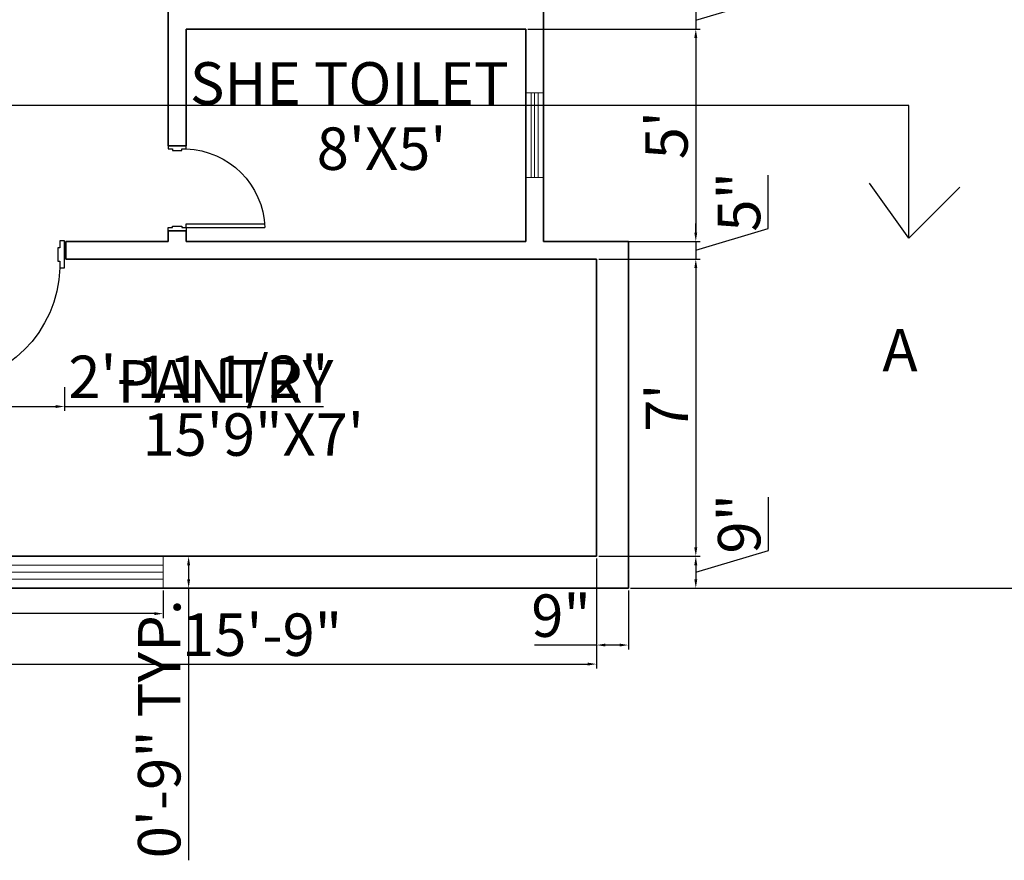
# Model space of a CAD drawing. Units: inches. Extents: x 2319 to 3765, y 2872 to 3950.
# Tile 5 of 9: x 2783 to 3061, y 2884 to 3121. Entities that reach past the tile are written whole.
import ezdxf

# ---------------------------------------------------------------- set-up
doc = ezdxf.new("R2010")
doc.units = ezdxf.units.IN
for name, color, linetype, lineweight in [('A-ANNO-DIMS', 2, 'Continuous', 18), ('A-ANNO-SYMB', 3, 'Continuous', 25), ('A-AREA-IDEN', 7, 'Continuous', 18), ('A-DOOR', 3, 'Continuous', 25), ('A-FURN', 8, 'Continuous', 18), ('A-GLAZ', 4, 'Continuous', 18), ('A-WALL', 7, 'Continuous', 35)]:
    doc.layers.add(name, color=color, linetype=linetype, lineweight=lineweight)
doc.styles.get("Standard").update_dxf_attribs({"font": 'arial.ttf'})
doc.dimstyles.new('ISO-25', dxfattribs={"dimtxt": 12, "dimasz": 2.5, "dimexe": 1.25, "dimexo": 0.625, "dimtad": 1, "dimdec": 0, "dimlunit": 3, "dimtxsty": 'Standard', "dimcen": 2.5, "dimadec": 0, "dimazin": 0, "dimtfac": 1, "dimtdec": 0, "dimtmove": 0, "dimatfit": 3, "dimfxl": 1, "dimarcsym": 0})

# ---------------------------------------------------------------- blocks, each defined once
blk = doc.blocks.new('A$C769D55ED')
for p, q in [((33.6, 192), (33.6, 1024.8)), ((72, 192), (72, 1023.9)), ((0, 192), (0, 0)), ((33.6, 192), (0, 192)), ((33.6, 144), (33.6, 192)), ((48, 144), (33.6, 144)), ((48, 48), (48, 144)), ((33.6, 0), (33.6, 48)), ((33.6, 48), (48, 48)), ((0, 0), (33.6, 0))]:
    blk.add_line(p, q)
blk.add_lwpolyline([(33.6, 192), (72, 192)])
blk.add_lwpolyline([(900, 192), (900, 0), (866.4, 0), (866.4, 48), (852, 48), (852, 144), (866.4, 144), (866.4, 192)], close=True)
blk.add_arc((7.2, 165.6), 859.6, 1.76235, 88.23765)
blk = doc.blocks.new('A$C0EDB4AB9')
at = {"linetype": 'ByBlock'}
for p, q in [((1257, 3447), (1257, 3084)), ((1303, 3447), (1257, 3447)), ((1303, 3084), (1303, 3447)), ((1342, 3055), (1342, 3493)), ((1842, 3493), (1842, 3051)), ((1873, 3447), (1873, 3084)), ((1919, 3447), (1873, 3447)), ((1919, 3084), (1919, 3447)), ((2028, 3447), (2028, 3084)), ((2074, 3447), (2028, 3447)), ((2074, 3084), (2074, 3447)), ((2114, 3055), (2114, 3493)), ((2614, 3493), (2614, 3051)), ((2644, 3447), (2644, 3084)), ((2691, 3447), (2644, 3447)), ((2691, 3084), (2691, 3447)), ((2790, 3447), (2790, 3084)), ((2836, 3447), (2790, 3447)), ((2836, 3084), (2836, 3447)), ((2875, 3055), (2875, 3493)), ((3375, 3493), (3375, 3051)), ((3406, 3447), (3406, 3084)), ((3452, 3447), (3406, 3447)), ((3452, 3084), (3452, 3447)), ((3537, 3447), (3537, 3084)), ((3583, 3447), (3537, 3447)), ((3583, 3084), (3583, 3447)), ((3622, 3055), (3622, 3493)), ((4122, 3493), (4122, 3051)), ((4153, 3447), (4153, 3084)), ((4199, 3447), (4153, 3447)), ((4199, 3084), (4199, 3447)), ((4314, 3447), (4314, 3084)), ((4360, 3447), (4314, 3447)), ((4360, 3084), (4360, 3447)), ((4399, 3055), (4399, 3493)), ((4899, 3493), (4899, 3051)), ((4930, 3447), (4930, 3084)), ((4976, 3447), (4930, 3447)), ((4976, 3084), (4976, 3447)), ((5158, 3447), (5158, 3084)), ((5204, 3447), (5158, 3447)), ((5204, 3084), (5204, 3447)), ((5243, 3055), (5243, 3493)), ((5743, 3493), (5743, 3051)), ((5774, 3447), (5774, 3084)), ((5820, 3447), (5774, 3447)), ((5820, 3084), (5820, 3447)), ((5991, 3447), (5991, 3084)), ((6037, 3447), (5991, 3447)), ((6037, 3084), (6037, 3447)), ((6076, 3055), (6076, 3493)), ((6576, 3493), (6576, 3051)), ((6607, 3447), (6607, 3084)), ((6653, 3447), (6607, 3447)), ((6653, 3084), (6653, 3447)), ((770, 3117), (1098, 2820)), ((855, 3143), (824, 3109)), ((824, 3109), (1094, 2865)), ((1124, 2900), (855, 3143)), ((7050, 3209), (6772, 2975)), ((6802, 2940), (7080, 3173)), ((6804, 2891), (7139, 3172)), ((7080, 3173), (7050, 3209)), ((1257, 3084), (1303, 3084)), ((1772, 2993), (1413, 2995)), ((1791, 2993), (1772, 2993)), ((1873, 3084), (1919, 3084)), ((2028, 3084), (2074, 3084)), ((2544, 2993), (2185, 2995)), ((2562, 2993), (2544, 2993)), ((2644, 3084), (2691, 3084)), ((2790, 3084), (2836, 3084)), ((3305, 2993), (2946, 2995)), ((3324, 2993), (3305, 2993)), ((3406, 3084), (3452, 3084)), ((3537, 3084), (3583, 3084)), ((4052, 2993), (3693, 2995)), ((4070, 2993), (4052, 2993)), ((4153, 3084), (4199, 3084)), ((4314, 3084), (4360, 3084)), ((4829, 2993), (4470, 2995)), ((4847, 2993), (4829, 2993)), ((4930, 3084), (4976, 3084)), ((5158, 3084), (5204, 3084)), ((5673, 2993), (5314, 2995)), ((5692, 2993), (5673, 2993)), ((5774, 3084), (5820, 3084)), ((5991, 3084), (6037, 3084)), ((6506, 2993), (6147, 2995)), ((6525, 2993), (6506, 2993)), ((6607, 3084), (6653, 3084)), ((6772, 2975), (6802, 2940)), ((1094, 2865), (1124, 2900)), ((6056, 2871), (1856, 2871)), ((759, 2452), (435, 2746)), ((1094, 2729), (851, 2464)), ((1106, 2743), (1094, 2729)), ((7034, 2521), (6804, 2798)), ((7461, 2790), (7123, 2505)), ((7446, 2737), (7169, 2503)), ((7198, 2468), (7476, 2702)), ((7476, 2702), (7446, 2737)), ((442, 2687), (411, 2653)), ((411, 2653), (680, 2409)), ((711, 2443), (442, 2687)), ((680, 2409), (711, 2443)), ((7169, 2503), (7198, 2468)), ((608, 2159), (245, 2159)), ((245, 2159), (245, 2113)), ((608, 2113), (608, 2159)), ((7619, 2213), (7256, 2213)), ((7256, 2213), (7256, 2167)), ((7256, 2167), (7619, 2167)), ((7619, 2167), (7619, 2213)), ((200, 2082), (642, 2082)), ((245, 2113), (608, 2113)), ((700, 2031), (700, 2012)), ((7165, 1697), (7167, 2056)), ((7227, 2127), (7665, 2127)), ((700, 2012), (698, 1653)), ((7165, 1679), (7165, 1697)), ((7665, 1627), (7223, 1627)), ((638, 1582), (200, 1582)), ((608, 1543), (245, 1543)), ((245, 1543), (245, 1497)), ((245, 1497), (608, 1497)), ((608, 1497), (608, 1543)), ((7619, 1597), (7256, 1597)), ((7256, 1597), (7256, 1550)), ((7256, 1550), (7619, 1550)), ((7619, 1550), (7619, 1597)), ((748, 1304), (442, 1107)), ((446, 1018), (817, 1257)), ((467, 1068), (772, 1265)), ((772, 1265), (748, 1304)), ((894, 1245), (904, 1230)), ((904, 1230), (1097, 927)), ((6802, 1000), (7057, 1253)), ((7150, 1260), (7459, 951)), ((7231, 1300), (7198, 1267)), ((7198, 1267), (7455, 1011)), ((7487, 1043), (7231, 1300)), ((442, 1107), (467, 1068)), ((6788, 987), (6802, 1000)), ((7455, 1011), (7487, 1043)), ((1084, 834), (716, 598)), ((6056, 871), (1856, 871)), ((6795, 864), (6763, 831)), ((6763, 831), (7019, 575)), ((7106, 597), (6793, 909)), ((7052, 607), (6795, 864)), ((1081, 786), (776, 589)), ((800, 550), (1106, 747)), ((1106, 747), (1081, 786)), ((1352, 723), (1370, 723)), ((1370, 723), (1730, 722)), ((2218, 723), (2236, 723)), ((2236, 723), (2595, 722)), ((2986, 700), (3005, 700)), ((3005, 700), (3364, 698)), ((3827, 723), (3846, 723)), ((3846, 723), (4205, 722)), ((4589, 723), (4607, 723)), ((4607, 723), (4966, 722)), ((5335, 723), (5354, 723)), ((5354, 723), (5713, 722)), ((6131, 723), (6149, 723)), ((6149, 723), (6508, 722)), ((776, 589), (800, 550)), ((1270, 632), (1224, 632)), ((1224, 632), (1224, 269)), ((1270, 269), (1270, 632)), ((1300, 223), (1300, 665)), ((1800, 661), (1800, 223)), ((1886, 632), (1840, 632)), ((1840, 632), (1840, 269)), ((1886, 269), (1886, 632)), ((2135, 632), (2089, 632)), ((2089, 632), (2089, 269)), ((2135, 269), (2135, 632)), ((2166, 223), (2166, 665)), ((2666, 661), (2666, 223)), ((2752, 632), (2705, 632)), ((2705, 632), (2705, 269)), ((2752, 269), (2752, 632)), ((2904, 608), (2858, 608)), ((2858, 608), (2858, 245)), ((2904, 245), (2904, 608)), ((2935, 200), (2935, 642)), ((3435, 638), (3435, 200)), ((3520, 608), (3474, 608)), ((3474, 608), (3474, 245)), ((3520, 245), (3520, 608)), ((3745, 632), (3699, 632)), ((3699, 632), (3699, 269)), ((3745, 269), (3745, 632)), ((3776, 223), (3776, 665)), ((4276, 661), (4276, 223)), ((4361, 632), (4315, 632)), ((4315, 632), (4315, 269)), ((4361, 269), (4361, 632)), ((4507, 632), (4461, 632)), ((4461, 632), (4461, 269)), ((4507, 269), (4507, 632)), ((4537, 223), (4537, 665)), ((5037, 661), (5037, 223)), ((5123, 632), (5077, 632)), ((5077, 632), (5077, 269)), ((5123, 269), (5123, 632)), ((5253, 632), (5207, 632)), ((5207, 632), (5207, 269)), ((5253, 269), (5253, 632)), ((5284, 223), (5284, 665)), ((5784, 661), (5784, 223)), ((5869, 632), (5823, 632)), ((5823, 632), (5823, 269)), ((5869, 269), (5869, 632)), ((6049, 632), (6003, 632)), ((6003, 632), (6003, 269)), ((6049, 269), (6049, 632)), ((6079, 223), (6079, 665)), ((6579, 661), (6579, 223)), ((6665, 632), (6619, 632)), ((6619, 632), (6619, 269)), ((6665, 269), (6665, 632)), ((7019, 575), (7052, 607)), ((1224, 269), (1270, 269)), ((1840, 269), (1886, 269)), ((2089, 269), (2135, 269)), ((2705, 269), (2752, 269)), ((2858, 245), (2904, 245)), ((3474, 245), (3520, 245)), ((3699, 269), (3745, 269)), ((4315, 269), (4361, 269)), ((4461, 269), (4507, 269)), ((5077, 269), (5123, 269)), ((5207, 269), (5253, 269)), ((5823, 269), (5869, 269)), ((6003, 269), (6049, 269)), ((6619, 269), (6665, 269))]:
    blk.add_line(p, q, dxfattribs=at)
for centre, radius, start, end in [((1592, 3230), 463, 52.6032, 130.8409), ((2364, 3230), 463, 52.6032, 130.8409), ((3125, 3230), 463, 52.6032, 130.8409), ((3872, 3230), 463, 52.6032, 130.8409), ((4649, 3230), 463, 52.6032, 130.8409), ((5493, 3230), 463, 52.6032, 130.8409), ((6326, 3230), 463, 52.6032, 130.8409), ((1335, 3551), 50, 127.3845, 320.4832), ((1592, 3230), 363, 46.3972, 133.6028), ((1837, 3560), 50, 219.1941, 46.1701), ((2107, 3551), 50, 127.3845, 320.4832), ((2364, 3230), 363, 46.3972, 133.6028), ((2609, 3560), 50, 219.1941, 46.1701), ((2869, 3551), 50, 127.3845, 320.4832), ((3125, 3230), 363, 46.3972, 133.6028), ((3370, 3560), 50, 219.1941, 46.1701), ((3615, 3551), 50, 127.3845, 320.4832), ((3872, 3230), 363, 46.3972, 133.6028), ((4117, 3560), 50, 219.1941, 46.1701), ((4392, 3551), 50, 127.3845, 320.4832), ((4649, 3230), 363, 46.3972, 133.6028), ((4894, 3560), 50, 219.1941, 46.1701), ((5236, 3551), 50, 127.3845, 320.4832), ((5493, 3230), 363, 46.3972, 133.6028), ((5738, 3560), 50, 219.1941, 46.1701), ((6069, 3551), 50, 127.3845, 320.4832), ((6326, 3230), 363, 46.3972, 133.6028), ((6571, 3560), 50, 219.1941, 46.1701), ((7180, 3215), 50, 77.4483, 270.5471), ((7100, 2812), 463, 2.6671, 80.9047), ((797, 2755), 463, 100.4356, 178.6733), ((797, 2755), 363, 94.2296, 181.4352), ((717, 3158), 50, 267.0265, 94.0025), ((7100, 2812), 363, 356.461, 83.6667), ((1412, 3065), 70.2, 172.0281, 271.1673), ((1782, 3053), 60.7, 261.2421, 1.6502), ((2183, 3065), 70.2, 172.0281, 271.1673), ((2553, 3053), 60.7, 261.2421, 1.6502), ((2945, 3065), 70.2, 172.0281, 271.1673), ((3315, 3053), 60.7, 261.2421, 1.6502), ((3691, 3065), 70.2, 172.0281, 271.1673), ((4061, 3053), 60.7, 261.2421, 1.6502), ((4468, 3065), 70.2, 172.0281, 271.1673), ((4838, 3053), 60.7, 261.2421, 1.6502), ((5313, 3065), 70.2, 172.0281, 271.1673), ((5682, 3053), 60.7, 261.2421, 1.6502), ((6146, 3065), 70.2, 172.0281, 271.1673), ((6515, 3053), 60.7, 261.2421, 1.6502), ((1856, 1871), 1000, 90, 270), ((6056, 1871), 1000, 270, 90), ((6857, 2844), 70.2, 122.0919, 221.2312), ((7510, 2837), 50, 169.258, 356.234), ((386, 2780), 50, 175.2169, 8.3156), ((1056, 2776), 60.7, 309.0745, 49.4826), ((798, 2510), 70.2, 219.8605, 318.9997), ((7083, 2551), 60.7, 211.3059, 311.714), ((7723, 2134), 50, 37.3845, 230.4832), ((7402, 1877), 463, 322.6032, 40.8409), ((462, 1832), 463, 142.6032, 220.8409), ((132, 2077), 50, 309.1941, 136.1701), ((462, 1832), 363, 136.3972, 223.6028), ((640, 2021), 60.7, 351.2421, 91.6502), ((7237, 2058), 70.2, 82.0281, 181.1673), ((7402, 1877), 363, 316.3972, 43.6028), ((628, 1651), 70.2, 262.0281, 1.1673), ((7225, 1688), 60.7, 171.2421, 271.6502), ((7732, 1632), 50, 129.1941, 316.1701), ((141, 1575), 50, 217.3845, 50.4832), ((848, 1205), 60.7, 24.0035, 124.4116), ((7107, 1204), 70.2, 37.0567, 136.1959), ((802, 950), 463, 175.3647, 253.6023), ((392, 977), 50, 341.9556, 168.9315), ((802, 950), 363, 169.1586, 256.3643), ((6837, 951), 60.7, 126.2707, 226.6788), ((7097, 960), 363, 271.4258, 358.6314), ((7506, 914), 50, 352.4131, 185.5118), ((1039, 888), 70.2, 294.7895, 33.9288), ((7097, 960), 463, 277.6319, 355.8695), ((1361, 663), 60.7, 81.2421, 181.6502), ((1731, 651), 70.2, 352.0281, 91.1673), ((2227, 663), 60.7, 81.2421, 181.6502), ((2597, 651), 70.2, 352.0281, 91.1673), ((2996, 640), 60.7, 81.2421, 181.6502), ((3365, 628), 70.2, 352.0281, 91.1673), ((3836, 663), 60.7, 81.2421, 181.6502), ((4206, 651), 70.2, 352.0281, 91.1673), ((4598, 663), 60.7, 81.2421, 181.6502), ((4968, 651), 70.2, 352.0281, 91.1673), ((5345, 663), 60.7, 81.2421, 181.6502), ((5714, 651), 70.2, 352.0281, 91.1673), ((6140, 663), 60.7, 81.2421, 181.6502), ((6510, 651), 70.2, 352.0281, 91.1673), ((671, 560), 50, 250.1459, 83.2447), ((7157, 553), 50, 84.2228, 271.1987), ((1306, 156), 50, 39.1941, 226.1701), ((1550, 486), 463, 232.6032, 310.8409), ((1550, 486), 363, 226.3972, 313.6028), ((1807, 165), 50, 307.3845, 140.4832), ((2171, 156), 50, 39.1941, 226.1701), ((2416, 486), 463, 232.6032, 310.8409), ((2416, 486), 363, 226.3972, 313.6028), ((2673, 165), 50, 307.3845, 140.4832), ((2940, 132), 50, 39.1941, 226.1701), ((3185, 462), 363, 226.3972, 313.6028), ((3442, 141), 50, 307.3845, 140.4832), ((3781, 156), 50, 39.1941, 226.1701), ((4026, 486), 463, 232.6032, 310.8409), ((4026, 486), 363, 226.3972, 313.6028), ((4283, 165), 50, 307.3845, 140.4832), ((4543, 156), 50, 39.1941, 226.1701), ((4787, 486), 463, 232.6032, 310.8409), ((4787, 486), 363, 226.3972, 313.6028), ((5044, 165), 50, 307.3845, 140.4832), ((5289, 156), 50, 39.1941, 226.1701), ((5534, 486), 463, 232.6032, 310.8409), ((5534, 486), 363, 226.3972, 313.6028), ((5791, 165), 50, 307.3845, 140.4832), ((6084, 156), 50, 39.1941, 226.1701), ((6329, 486), 463, 232.6032, 310.8409), ((6329, 486), 363, 226.3972, 313.6028), ((6586, 165), 50, 307.3845, 140.4832), ((3185, 462), 463, 232.6032, 310.8409)]:
    blk.add_arc(centre, radius, start, end, dxfattribs=at)
blk = doc.blocks.new('*D15')
at = {"layer": 'A-ANNO-DIMS', "color": 0, "lineweight": -2, "transparency": 16777216}
for p, q in [((2994.67, 3127.26), (2994.67, 3142.3)), ((2974.18, 3126.11), (2974.18, 3128.61)), ((2974.18, 3121.11), (2994.67, 3127.26)), ((2926.75, 3123.61), (2975.43, 3123.61)), ((2974.18, 3123.61), (2974.18, 3118.61)), ((2974.18, 3123.61), (2974.18, 3118.61)), ((2926.75, 3118.61), (2975.43, 3118.61)), ((2974.18, 3116.11), (2974.18, 3113.61))]:
    blk.add_line(p, q, dxfattribs=at)
at = {"layer": 'A-ANNO-DIMS', "color": 0, "transparency": 16777216}
for points in [[(2973.76, 3126.11), (2974.59, 3126.11), (2974.18, 3123.61)], [(2973.76, 3116.11), (2974.59, 3116.11), (2974.18, 3118.61)]]:
    blk.add_solid(points, dxfattribs=at)
at = {"layer": 'Defpoints', "color": 0, "transparency": 16777216}
for p in [(2926.13, 3123.61), (2926.13, 3118.61), (2974.18, 3118.61)]:
    blk.add_point(p, dxfattribs=at)
at = {"layer": 'A-ANNO-DIMS', "color": 0, "transparency": 16777216, "insert": (2987.94, 3134.78), "char_height": 12, "attachment_point": 5, "rotation": 90}
blk.add_mtext('5"', dxfattribs=at)
blk = doc.blocks.new('*D16')
at = {"layer": 'A-ANNO-DIMS', "color": 0, "lineweight": -2, "transparency": 16777216}
for p, q in [((2926.75, 3118.61), (2975.43, 3118.61)), ((2974.18, 3116.11), (2974.18, 3061.11)), ((2931.75, 3058.61), (2975.43, 3058.61))]:
    blk.add_line(p, q, dxfattribs=at)
at = {"layer": 'A-ANNO-DIMS', "color": 0, "transparency": 16777216}
for points in [[(2973.76, 3116.11), (2974.59, 3116.11), (2974.18, 3118.61)], [(2973.76, 3061.11), (2974.59, 3061.11), (2974.18, 3058.61)]]:
    blk.add_solid(points, dxfattribs=at)
at = {"layer": 'Defpoints', "color": 0, "transparency": 16777216}
for p in [(2926.13, 3118.61), (2931.13, 3058.61), (2974.18, 3058.61)]:
    blk.add_point(p, dxfattribs=at)
at = {"layer": 'A-ANNO-DIMS', "color": 0, "transparency": 16777216, "insert": (2967.45, 3088.61), "char_height": 12, "attachment_point": 5, "rotation": 90}
blk.add_mtext("5'", dxfattribs=at)
blk = doc.blocks.new('*D17')
at = {"layer": 'A-ANNO-DIMS', "color": 0, "lineweight": -2, "transparency": 16777216}
for p, q in [((2994.67, 3062.26), (2994.67, 3077.3)), ((2974.18, 3061.11), (2974.18, 3063.61)), ((2974.18, 3056.11), (2994.67, 3062.26)), ((2931.75, 3058.61), (2975.43, 3058.61)), ((2974.18, 3058.61), (2974.18, 3053.61)), ((2974.18, 3058.61), (2974.18, 3053.61)), ((2946.75, 3053.61), (2975.43, 3053.61)), ((2974.18, 3051.11), (2974.18, 3048.61))]:
    blk.add_line(p, q, dxfattribs=at)
at = {"layer": 'A-ANNO-DIMS', "color": 0, "transparency": 16777216}
for points in [[(2973.76, 3061.11), (2974.59, 3061.11), (2974.18, 3058.61)], [(2973.76, 3051.11), (2974.59, 3051.11), (2974.18, 3053.61)]]:
    blk.add_solid(points, dxfattribs=at)
at = {"layer": 'Defpoints', "color": 0, "transparency": 16777216}
for p in [(2931.13, 3058.61), (2946.13, 3053.61), (2974.18, 3053.61)]:
    blk.add_point(p, dxfattribs=at)
at = {"layer": 'A-ANNO-DIMS', "color": 0, "transparency": 16777216, "insert": (2987.94, 3069.78), "char_height": 12, "attachment_point": 5, "rotation": 90}
blk.add_mtext('5"', dxfattribs=at)
blk = doc.blocks.new('*D18')
at = {"layer": 'A-ANNO-DIMS', "color": 0, "lineweight": -2, "transparency": 16777216}
for p, q in [((2946.75, 3053.61), (2975.43, 3053.61)), ((2974.18, 3051.11), (2974.18, 2972.11)), ((2946.75, 2969.61), (2975.43, 2969.61))]:
    blk.add_line(p, q, dxfattribs=at)
at = {"layer": 'A-ANNO-DIMS', "color": 0, "transparency": 16777216}
for points in [[(2973.76, 3051.11), (2974.59, 3051.11), (2974.18, 3053.61)], [(2973.76, 2972.11), (2974.59, 2972.11), (2974.18, 2969.61)]]:
    blk.add_solid(points, dxfattribs=at)
at = {"layer": 'Defpoints', "color": 0, "transparency": 16777216}
for p in [(2946.13, 3053.61), (2946.13, 2969.61), (2974.18, 2969.61)]:
    blk.add_point(p, dxfattribs=at)
at = {"layer": 'A-ANNO-DIMS', "color": 0, "transparency": 16777216, "insert": (2967.55, 3011.61), "char_height": 12, "attachment_point": 5, "rotation": 90}
blk.add_mtext("7'", dxfattribs=at)
blk = doc.blocks.new('*D19')
at = {"layer": 'A-ANNO-DIMS', "color": 0, "lineweight": -2, "transparency": 16777216}
for p, q in [((2994.74, 2971.28), (2994.74, 2986.32)), ((2946.75, 2969.61), (2975.43, 2969.61)), ((2974.18, 2965.11), (2994.74, 2971.28)), ((2974.18, 2967.11), (2974.18, 2963.11)), ((2955.75, 2960.61), (2975.43, 2960.61))]:
    blk.add_line(p, q, dxfattribs=at)
at = {"layer": 'A-ANNO-DIMS', "color": 0, "transparency": 16777216}
for points in [[(2973.76, 2967.11), (2974.59, 2967.11), (2974.18, 2969.61)], [(2973.76, 2963.11), (2974.59, 2963.11), (2974.18, 2960.61)]]:
    blk.add_solid(points, dxfattribs=at)
at = {"layer": 'Defpoints', "color": 0, "transparency": 16777216}
for p in [(2946.13, 2969.61), (2955.13, 2960.61), (2974.18, 2960.61)]:
    blk.add_point(p, dxfattribs=at)
at = {"layer": 'A-ANNO-DIMS', "color": 0, "transparency": 16777216, "insert": (2987.99, 2978.8), "char_height": 12, "attachment_point": 5, "rotation": 90}
blk.add_mtext('9"', dxfattribs=at)
blk = doc.blocks.new('*D22')
at = {"layer": 'A-ANNO-DIMS', "color": 0, "lineweight": -2, "transparency": 16777216}
for p, q in [((2757.13, 2968.99), (2757.13, 2937.91)), ((2946.13, 2968.99), (2946.13, 2937.91)), ((2759.63, 2939.16), (2943.63, 2939.16))]:
    blk.add_line(p, q, dxfattribs=at)
at = {"layer": 'A-ANNO-DIMS', "color": 0, "transparency": 16777216}
for points in [[(2759.63, 2939.58), (2759.63, 2938.74), (2757.13, 2939.16)], [(2943.63, 2939.58), (2943.63, 2938.74), (2946.13, 2939.16)]]:
    blk.add_solid(points, dxfattribs=at)
at = {"layer": 'Defpoints', "color": 0, "transparency": 16777216}
for p in [(2757.13, 2969.61), (2946.13, 2969.61), (2946.13, 2939.16)]:
    blk.add_point(p, dxfattribs=at)
at = {"layer": 'A-ANNO-DIMS', "color": 0, "transparency": 16777216, "insert": (2851.63, 2945.91), "char_height": 12, "attachment_point": 5}
blk.add_mtext('15\'-9"', dxfattribs=at)
blk = doc.blocks.new('*D26')
at = {"layer": 'A-ANNO-DIMS', "color": 0, "lineweight": -2, "transparency": 16777216}
for p, q in [((2955.13, 2959.99), (2955.13, 2943.29)), ((2946.13, 2952.82), (2946.13, 2943.29)), ((2946.13, 2944.54), (2928.58, 2944.54)), ((2952.63, 2944.54), (2948.63, 2944.54))]:
    blk.add_line(p, q, dxfattribs=at)
at = {"layer": 'A-ANNO-DIMS', "color": 0, "transparency": 16777216}
for points in [[(2948.63, 2944.95), (2948.63, 2944.12), (2946.13, 2944.54)], [(2952.63, 2944.95), (2952.63, 2944.12), (2955.13, 2944.54)]]:
    blk.add_solid(points, dxfattribs=at)
at = {"layer": 'Defpoints', "color": 0, "transparency": 16777216}
for p in [(2955.13, 2960.61), (2946.13, 2953.45), (2946.13, 2944.54)]:
    blk.add_point(p, dxfattribs=at)
at = {"layer": 'A-ANNO-DIMS', "color": 0, "transparency": 16777216, "insert": (2936.11, 2951.29), "char_height": 12, "attachment_point": 5}
blk.add_mtext('9"', dxfattribs=at)
blk = doc.blocks.new('WIN-48-PLAN-9IN-WALL')
for p, q in [((0, 9), (0, 0)), ((48, 9), (48, 0)), ((48, 6.5), (0, 6.5)), ((48, 4.5), (0, 4.5)), ((48, 2.5), (0, 2.5))]:
    blk.add_line(p, q)
blk = doc.blocks.new('WIN-24-PLAN-5IN-WALL')
for p, q in [((0, 24), (5, 24)), ((1.5, 0), (1.5, 24)), ((2.5, 0), (2.5, 24)), ((3.5, 0), (3.5, 24)), ((0, 0), (5, 0))]:
    blk.add_line(p, q)
blk = doc.blocks.new('SECTION-ARROWHEAD')
for q in [(0, 15.55), (25.55, 14.43)]:
    blk.add_line((11.08, 0), q)
blk = doc.blocks.new('*D52')
at = {"layer": 'A-ANNO-DIMS', "color": 0, "lineweight": -2, "transparency": 16777216}
for p, q in [((2760.07, 3017.41), (2760.07, 3010.68)), ((2795.8, 3017.41), (2795.8, 3010.68)), ((2762.57, 3011.93), (2793.3, 3011.93)), ((2795.8, 3011.93), (2868.94, 3011.93))]:
    blk.add_line(p, q, dxfattribs=at)
at = {"layer": 'A-ANNO-DIMS', "color": 0, "transparency": 16777216}
for points in [[(2762.57, 3012.35), (2762.57, 3011.52), (2760.07, 3011.93)], [(2793.3, 3012.35), (2793.3, 3011.52), (2795.8, 3011.93)]]:
    blk.add_solid(points, dxfattribs=at)
at = {"layer": 'Defpoints', "color": 0, "transparency": 16777216}
for p in [(2760.07, 3018.04), (2795.8, 3018.04), (2795.8, 3011.93)]:
    blk.add_point(p, dxfattribs=at)
at = {"layer": 'A-ANNO-DIMS', "color": 0, "transparency": 16777216, "insert": (2833.62, 3018.76), "char_height": 12, "attachment_point": 5}
blk.add_mtext('2\'-11 1/2"', dxfattribs=at)
blk = doc.blocks.new('*D59')
at = {"layer": 'A-ANNO-DIMS', "color": 0, "lineweight": -2, "transparency": 16777216}
for p, q in [((2775.67, 2959.99), (2775.67, 2952.16)), ((2823.67, 2959.99), (2823.67, 2952.16)), ((2775.67, 2953.41), (2620.07, 2953.41)), ((2821.17, 2953.41), (2778.17, 2953.41))]:
    blk.add_line(p, q, dxfattribs=at)
at = {"layer": 'A-ANNO-DIMS', "color": 0, "transparency": 16777216}
for points in [[(2778.17, 2953.83), (2778.17, 2952.99), (2775.67, 2953.41)], [(2821.17, 2953.83), (2821.17, 2952.99), (2823.67, 2953.41)]]:
    blk.add_solid(points, dxfattribs=at)
at = {"layer": 'Defpoints', "color": 0, "transparency": 16777216}
for p in [(2775.67, 2960.61), (2823.67, 2960.61), (2775.67, 2953.41)]:
    blk.add_point(p, dxfattribs=at)
at = {"layer": 'A-ANNO-DIMS', "color": 0, "transparency": 16777216, "insert": (2696.62, 2960.24), "char_height": 12, "attachment_point": 5}
blk.add_mtext('WINDOW 4\'-0" TYP.', dxfattribs=at)
blk = doc.blocks.new('*D60')
at = {"layer": 'A-ANNO-DIMS', "color": 0, "lineweight": -2, "transparency": 16777216}
for p, q in [((2824.29, 2969.61), (2832.12, 2969.61)), ((2830.87, 2967.11), (2830.87, 2963.11)), ((2824.29, 2960.61), (2832.12, 2960.61)), ((2830.87, 2960.61), (2830.87, 2883.71))]:
    blk.add_line(p, q, dxfattribs=at)
at = {"layer": 'A-ANNO-DIMS', "color": 0, "transparency": 16777216}
for points in [[(2830.45, 2967.11), (2831.28, 2967.11), (2830.87, 2969.61)], [(2830.45, 2963.11), (2831.28, 2963.11), (2830.87, 2960.61)]]:
    blk.add_solid(points, dxfattribs=at)
at = {"layer": 'Defpoints', "color": 0, "transparency": 16777216}
for p in [(2823.67, 2969.61), (2823.67, 2960.61), (2830.87, 2960.61)]:
    blk.add_point(p, dxfattribs=at)
at = {"layer": 'A-ANNO-DIMS', "color": 0, "transparency": 16777216, "insert": (2824.11, 2920.91), "char_height": 12, "attachment_point": 5, "rotation": 90}
blk.add_mtext('0\'-9" TYP.', dxfattribs=at)
blk = doc.blocks.new('*D72')
at = {"layer": 'A-ANNO-DIMS', "color": 0, "lineweight": -2, "transparency": 16777216}
for p, q in [((2955.75, 3568.61), (3085.2, 3568.61)), ((3083.95, 2963.11), (3083.95, 3566.11)), ((2955.75, 2960.61), (3085.2, 2960.61))]:
    blk.add_line(p, q, dxfattribs=at)
at = {"layer": 'A-ANNO-DIMS', "color": 0, "transparency": 16777216}
for points in [[(3083.53, 3566.11), (3084.36, 3566.11), (3083.95, 3568.61)], [(3083.53, 2963.11), (3084.36, 2963.11), (3083.95, 2960.61)]]:
    blk.add_solid(points, dxfattribs=at)
at = {"layer": 'Defpoints', "color": 0, "transparency": 16777216}
for p in [(2955.13, 3568.61), (3083.95, 3568.61), (2955.13, 2960.61)]:
    blk.add_point(p, dxfattribs=at)
at = {"layer": 'A-ANNO-DIMS', "color": 0, "transparency": 16777216, "insert": (3077.2, 3264.61), "char_height": 12, "attachment_point": 5, "rotation": 90}
blk.add_mtext('50\'-8"', dxfattribs=at)
blk = doc.blocks.new('*D76')
at = {"layer": 'A-ANNO-DIMS', "color": 0, "lineweight": -2, "transparency": 16777216}
for p, q in [((2757.13, 2970.24), (2757.13, 3605.01)), ((2759.63, 3603.76), (2773.17, 3603.76)), ((2775.67, 2970.24), (2775.67, 3605.01)), ((2775.67, 3603.76), (2838.15, 3603.76))]:
    blk.add_line(p, q, dxfattribs=at)
at = {"layer": 'A-ANNO-DIMS', "color": 0, "transparency": 16777216}
for points in [[(2759.63, 3604.18), (2759.63, 3603.34), (2757.13, 3603.76)], [(2773.17, 3604.18), (2773.17, 3603.34), (2775.67, 3603.76)]]:
    blk.add_solid(points, dxfattribs=at)
at = {"layer": 'Defpoints', "color": 0, "transparency": 16777216}
for p in [(2775.67, 3603.76), (2757.13, 2969.61), (2775.67, 2969.61)]:
    blk.add_point(p, dxfattribs=at)
at = {"layer": 'A-ANNO-DIMS', "color": 0, "transparency": 16777216, "insert": (2808.16, 3610.59), "char_height": 12, "attachment_point": 5}
blk.add_mtext('1\'-6 1/2"', dxfattribs=at)

msp = doc.modelspace()

# ---------------------------------------------------------------- linework, layer by layer
at = {"layer": 'A-ANNO-SYMB'}
for p, q in [((3034.33, 3097.01), (2389.37, 3097.01)), ((3034.33, 3059.5), (3034.33, 3097.01))]:
    msp.add_line(p, q, dxfattribs=at)
at = {"layer": 'A-WALL'}
for p, q in [((2931.13, 3058.61), (2931.13, 3248.61)), ((2825.13, 3085.61), (2825.13, 3126.61)), ((2926.13, 3118.61), (2830.13, 3118.61)), ((2830.13, 3085.61), (2830.13, 3118.61)), ((2926.13, 3058.61), (2926.13, 3118.61)), ((2830.13, 3085.61), (2825.13, 3085.61)), ((2830.13, 3061.61), (2825.13, 3061.61)), ((2825.13, 3058.61), (2825.13, 3061.61)), ((2830.13, 3058.61), (2830.13, 3061.61)), ((2825.13, 3058.61), (2796.13, 3058.61)), ((2796.13, 3058.61), (2796.13, 3053.61)), ((2926.13, 3058.61), (2830.13, 3058.61)), ((2955.13, 3058.61), (2931.13, 3058.61)), ((2955.13, 2960.61), (2955.13, 3058.61)), ((2946.13, 3053.61), (2796.13, 3053.61)), ((2946.13, 2969.61), (2946.13, 3053.61)), ((2757.13, 2969.61), (2946.13, 2969.61)), ((2474.13, 2960.61), (2955.13, 2960.61))]:
    msp.add_line(p, q, dxfattribs=at)

# ---------------------------------------------------------------- block references
at = {"layer": 'A-ANNO-SYMB'}
msp.add_blockref('SECTION-ARROWHEAD', (3023.25, 3059.5), dxfattribs=at)
at = {"layer": 'A-DOOR'}
for p, xscale, yscale, zscale, rotation in [((2825.07, 3061.61), -0.0266624880085475, 0.0266624880085475, 0.0266624880085475, 270), ((2760.07, 3058.72), -0.0397016870405166, 0.0397016870405166, 0.0397016870405166, 180)]:
    msp.add_blockref('A$C769D55ED', p, dxfattribs=dict(at, xscale=xscale, yscale=yscale, zscale=zscale, rotation=rotation))
at = {"layer": 'A-FURN', "xscale": 0.02062408179219, "yscale": 0.02062408179219, "zscale": 0.02062408179219}
msp.add_blockref('A$C0EDB4AB9', (2638.81, 3115.79), dxfattribs=at)
at = {"layer": 'A-GLAZ'}
msp.add_blockref('WIN-24-PLAN-5IN-WALL', (2926.13, 3076.61), dxfattribs=at)
at = {"layer": 'A-GLAZ', "rotation": 180}
msp.add_blockref('WIN-48-PLAN-9IN-WALL', (2823.67, 2969.61), dxfattribs=at)

# ---------------------------------------------------------------- texts
at = {"layer": 'A-ANNO-SYMB'}
msp.add_text('A', height=12, dxfattribs=at).set_placement((3026.91, 3021.89))
at = {"layer": 'A-AREA-IDEN'}
for s, p in [('SHE TOILET', (2831.23, 3097.23)), ("8'X5'", (2867.06, 3078.8)), ('PANTRY', (2810.74, 3013.06)), ('15\'9"X7\'', (2817.83, 2998.01))]:
    msp.add_text(s, height=12, dxfattribs=at).set_placement(p)

# ---------------------------------------------------------------- dimensions: what is measured, and where the dimension line sits
at = {"layer": 'A-ANNO-DIMS'}
for base, p1, p2, override, picture, middle in [((2775.67, 3603.76), (2757.13, 2969.61), (2775.67, 2969.61), {"dimdec": 1, "dimlfac": 1, "dimrnd": 0, "dimzin": 1, "dimdsep": 46, "dimlunit": 4, "dimfrac": 2}, '*D76', (2808.16, 3610.59)), ((2795.8, 3011.93), (2760.07, 3018.04), (2795.8, 3018.04), {"dimdec": 1, "dimlfac": 1, "dimrnd": 0, "dimzin": 1, "dimdsep": 46, "dimlunit": 4, "dimfrac": 2}, '*D52', (2833.62, 3018.76)), ((2946.13, 2939.16), (2757.13, 2969.61), (2946.13, 2969.61), {"dimclrd": 0, "dimclre": 0, "dimclrt": 0}, '*D22', (2851.63, 2945.91)), ((2946.13, 2944.54), (2955.13, 2960.61), (2946.13, 2953.45), {"dimclrd": 0, "dimclre": 0, "dimclrt": 0}, '*D26', (2936.11, 2951.29))]:
    dim = msp.add_linear_dim(base=base, p1=p1, p2=p2, dimstyle='ISO-25', override=override, dxfattribs=at)
    dim.commit()
    dim.dimension.update_dxf_attribs({"geometry": picture, "text_midpoint": middle})
for base, p1, p2, override, picture, middle in [((3083.95, 3568.61), (2955.13, 2960.61), (2955.13, 3568.61), {"dimdec": 1, "dimlfac": 1, "dimrnd": 0, "dimzin": 1, "dimdsep": 46, "dimlunit": 4, "dimfrac": 2}, '*D72', (3077.2, 3264.61)), ((2974.18, 3118.61), (2926.13, 3123.61), (2926.13, 3118.61), {"dimclrd": 0, "dimclre": 0, "dimclrt": 0, "dimtmove": 1}, '*D15', (2987.94, 3127.88)), ((2974.18, 3058.61), (2926.13, 3118.61), (2931.13, 3058.61), {"dimclrd": 0, "dimclre": 0, "dimclrt": 0, "dimtmove": 1}, '*D16', (2967.45, 3088.61)), ((2974.18, 3053.61), (2931.13, 3058.61), (2946.13, 3053.61), {"dimclrd": 0, "dimclre": 0, "dimclrt": 0, "dimtmove": 1}, '*D17', (2987.94, 3062.88)), ((2974.18, 2969.61), (2946.13, 3053.61), (2946.13, 2969.61), {"dimclrd": 0, "dimclre": 0, "dimclrt": 0, "dimtmove": 1}, '*D18', (2967.55, 3011.61)), ((2974.18, 2960.61), (2946.13, 2969.61), (2955.13, 2960.61), {"dimclrd": 0, "dimclre": 0, "dimclrt": 0, "dimtmove": 1}, '*D19', (2987.99, 2971.91))]:
    dim = msp.add_linear_dim(base=base, p1=p1, p2=p2, angle=90, dimstyle='ISO-25', override=override, dxfattribs=at)
    dim.commit()
    dim.dimension.update_dxf_attribs({"geometry": picture, "text_midpoint": middle})
for base, p1, p2, angle, text, picture, middle in [((2775.67, 2953.41), (2823.67, 2960.61), (2775.67, 2960.61), 180, 'WINDOW <> TYP.', '*D59', (2696.62, 2960.24)), ((2830.87, 2960.61), (2823.67, 2969.61), (2823.67, 2960.61), 270, '<> TYP.', '*D60', (2824.11, 2920.91))]:
    dim = msp.add_linear_dim(base=base, p1=p1, p2=p2, angle=angle, text=text, dimstyle='ISO-25', override={"dimdec": 1, "dimlfac": 1, "dimrnd": 0, "dimzin": 1, "dimdsep": 46, "dimlunit": 4, "dimfrac": 2}, dxfattribs=at)
    dim.commit()
    dim.dimension.update_dxf_attribs({"geometry": picture, "text_midpoint": middle})

doc.saveas('drawing.dxf')
